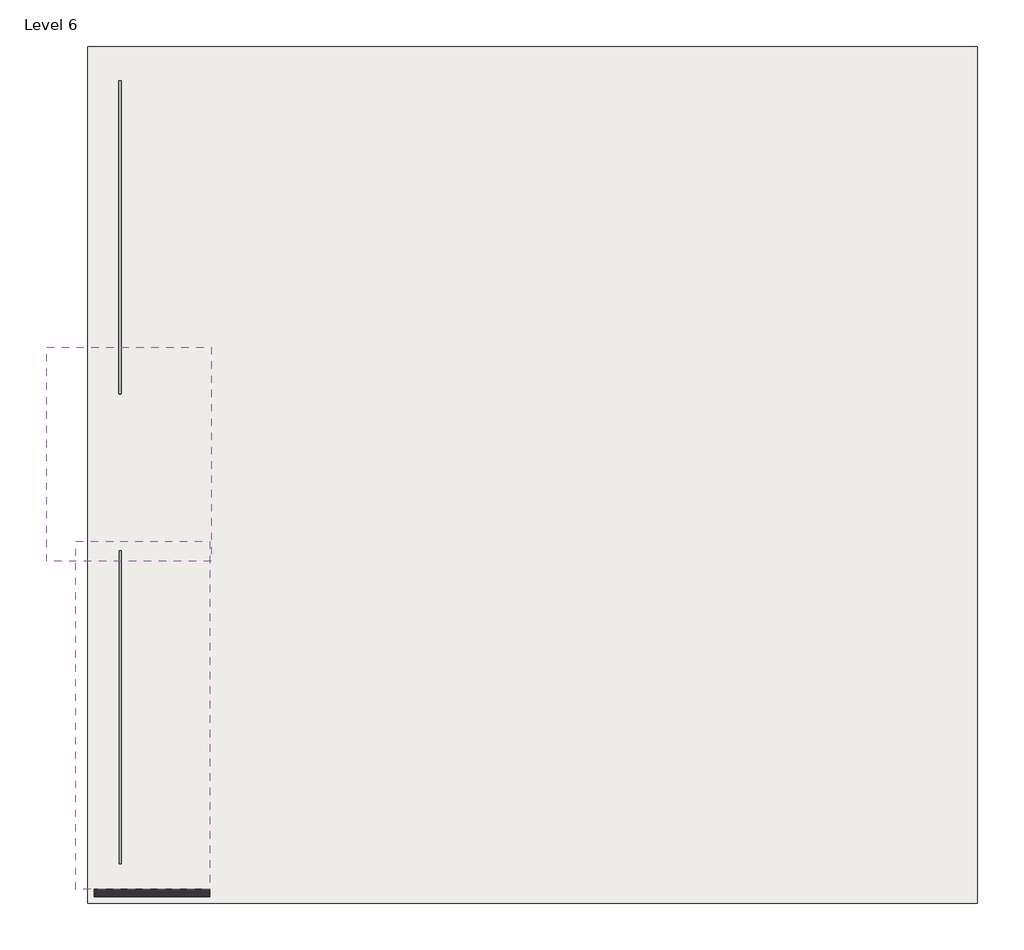
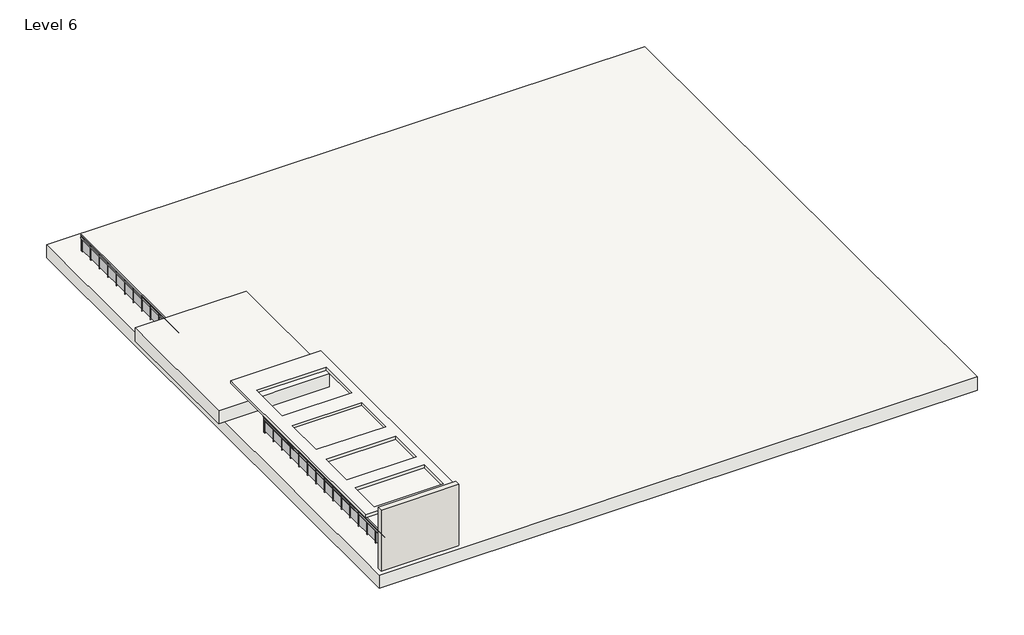
# One storey: 3 slabs, 2 railings, 1 wall.
"""IFC4 building model written with IfcOpenShell, lengths in millimetres."""

from ifc_helpers import new_model, si_unit, point, frame, origin, place, context, project, spatial, polyline, ellipse_curve, trimmed, outline, extrude, element, save
from ifc_brep_helpers import plane_surface, extruded_surface, advanced_brep

model = new_model("IFC4")

# Units and contexts
model_context = context("Model", 3, world=origin())
ifc_project = project(units=[si_unit("LENGTHUNIT", "METRE", prefix="MILLI")], contexts=[model_context])

# Site, building, storey
site = spatial("IfcSite", under=ifc_project)
building = spatial("IfcBuilding", under=site)
storey = spatial("IfcBuildingStorey", under=building, Name="Level 6", Elevation=15240.0)

# Railings
placement = place(None, origin())
element("IfcRailing", 1, ObjectType="Glass Panel - Bottom Fill", at=placement, inside=storey, context=model_context, shape_type="SolidModel", body=[
    advanced_brep(
    [(-15690.0723021, 14300.8556013, 16154.4), (-15766.2723021, 14300.8556013, 16154.4), (-15690.0723021, 2718.4556013, 16154.4), (-15766.2723021, 2718.4556013, 16154.4)],
    [
        (0, 1, ellipse_curve(frame((-15728.1723021, 14300.8556013, 16154.4), z_axis=(0.0, 1.0, 0.0), x_axis=(-1.0, 0.0, 0.0)), 38.1, 28.575)),
        (1, 0, ellipse_curve(frame((-15728.1723021, 14300.8556013, 16154.4), z_axis=(0.0, 1.0, 0.0), x_axis=(-1.0, 0.0, 0.0)), 38.1, 28.575)),
        (2, 3, ellipse_curve(frame((-15728.1723021, 2718.4556013, 16154.4), z_axis=(0.0, -1.0, 0.0), x_axis=(-1.0, 0.0, 0.0)), 38.1, 28.575)),
        (3, 2, ellipse_curve(frame((-15728.1723021, 2718.4556013, 16154.4), z_axis=(0.0, -1.0, 0.0), x_axis=(-1.0, 0.0, 0.0)), 38.1, 28.575)),
        (0, 2),
        (3, 1),
    ],
    [
        plane_surface(frame((-15728.1723021, 14300.8556013, 16154.4), z_axis=(0.0, 1.0, 0.0), x_axis=(0.0, 0.0, -1.0))),
        plane_surface(frame((-15728.1723021, 2718.4556013, 16154.4), z_axis=(0.0, -1.0, 0.0), x_axis=(0.0, 0.0, -1.0))),
        extruded_surface(trimmed(ellipse_curve(frame((-15728.1723021, 2718.4556013, 16154.4), z_axis=(0.0, 1.0, 0.0), x_axis=(-1.0, 0.0, 0.0)), 38.1, 28.575), [point((-15690.0723021, 2718.4556013, 16154.4))], [point((-15766.2723021, 2718.4556013, 16154.4))], True, "CARTESIAN"), (0.0, 11582.4, 0.0), 11582.4),
        extruded_surface(trimmed(ellipse_curve(frame((-15728.1723021, 2718.4556013, 16154.4), z_axis=(0.0, 1.0, 0.0), x_axis=(-1.0, 0.0, 0.0)), 38.1, 28.575), [point((-15766.2723021, 2718.4556013, 16154.4))], [point((-15690.0723021, 2718.4556013, 16154.4))], True, "CARTESIAN"), (0.0, 11582.4, 0.0), 11582.4),
    ],
    [
        (0, [[1, 2]]),
        (1, [[3, 4]]),
        (2, [[-1, 5, -4, 6]]),
        (3, [[-2, -6, -3, -5]]),
    ],
),
    extrude(outline(polyline([(-15753.5723021, 14300.8556013), (-15702.7723021, 14300.8556013), (-15702.7723021, 2718.4556013), (-15753.5723021, 2718.4556013), (-15753.5723021, 14300.8556013)])), frame((0.0, 0.0, 15976.6), z_axis=(0.0, 0.0, 1.0), x_axis=(1.0, 0.0, 0.0)), (0.0, 0.0, 1.0), 76.2),
    extrude(outline(polyline([(-15740.8723021, 14300.8556013), (-15715.4723021, 14300.8556013), (-15715.4723021, 2718.4556013), (-15740.8723021, 2718.4556013), (-15740.8723021, 14300.8556013)])), frame((0.0, 0.0, 15938.5), z_axis=(0.0, 0.0, 1.0), x_axis=(1.0, 0.0, 0.0)), (0.0, 0.0, 1.0), 25.4),
    extrude(outline(polyline([(-15753.5723021, 2826.4056013), (-15702.7723021, 2826.4056013), (-15702.7723021, 2813.7056013), (-15753.5723021, 2813.7056013), (-15753.5723021, 2826.4056013)])), frame((0.0, 0.0, 15240.0), z_axis=(0.0, 0.0, 1.0), x_axis=(1.0, 0.0, 0.0)), (0.0, 0.0, 1.0), 885.6788223),
    extrude(outline(polyline([(-15721.6371451, 3632.8556013), (-15721.6371451, 2820.0556013), (-15727.9871451, 2820.0556013), (-15727.9871451, 3632.8556013), (-15721.6371451, 3632.8556013)])), frame((0.0, 0.0, 15341.6), z_axis=(0.0, 0.0, 1.0), x_axis=(1.0, 0.0, 0.0)), (0.0, 0.0, 1.0), 596.9),
    extrude(outline(polyline([(-15753.5723021, 3639.2056013), (-15702.7723021, 3639.2056013), (-15702.7723021, 3626.5056013), (-15753.5723021, 3626.5056013), (-15753.5723021, 3639.2056013)])), frame((0.0, 0.0, 15240.0), z_axis=(0.0, 0.0, 1.0), x_axis=(1.0, 0.0, 0.0)), (0.0, 0.0, 1.0), 885.6788223),
    extrude(outline(polyline([(-15721.6371451, 4445.6556013), (-15721.6371451, 3632.8556013), (-15727.9871451, 3632.8556013), (-15727.9871451, 4445.6556013), (-15721.6371451, 4445.6556013)])), frame((0.0, 0.0, 15341.6), z_axis=(0.0, 0.0, 1.0), x_axis=(1.0, 0.0, 0.0)), (0.0, 0.0, 1.0), 596.9),
    extrude(outline(polyline([(-15753.5723021, 4452.0056013), (-15702.7723021, 4452.0056013), (-15702.7723021, 4439.3056013), (-15753.5723021, 4439.3056013), (-15753.5723021, 4452.0056013)])), frame((0.0, 0.0, 15240.0), z_axis=(0.0, 0.0, 1.0), x_axis=(1.0, 0.0, 0.0)), (0.0, 0.0, 1.0), 885.6788223),
    extrude(outline(polyline([(-15721.6371451, 5258.4556013), (-15721.6371451, 4445.6556013), (-15727.9871451, 4445.6556013), (-15727.9871451, 5258.4556013), (-15721.6371451, 5258.4556013)])), frame((0.0, 0.0, 15341.6), z_axis=(0.0, 0.0, 1.0), x_axis=(1.0, 0.0, 0.0)), (0.0, 0.0, 1.0), 596.9),
    extrude(outline(polyline([(-15753.5723021, 5264.8056013), (-15702.7723021, 5264.8056013), (-15702.7723021, 5252.1056013), (-15753.5723021, 5252.1056013), (-15753.5723021, 5264.8056013)])), frame((0.0, 0.0, 15240.0), z_axis=(0.0, 0.0, 1.0), x_axis=(1.0, 0.0, 0.0)), (0.0, 0.0, 1.0), 885.6788223),
    extrude(outline(polyline([(-15721.6371451, 6071.2556013), (-15721.6371451, 5258.4556013), (-15727.9871451, 5258.4556013), (-15727.9871451, 6071.2556013), (-15721.6371451, 6071.2556013)])), frame((0.0, 0.0, 15341.6), z_axis=(0.0, 0.0, 1.0), x_axis=(1.0, 0.0, 0.0)), (0.0, 0.0, 1.0), 596.9),
    extrude(outline(polyline([(-15753.5723021, 6077.6056013), (-15702.7723021, 6077.6056013), (-15702.7723021, 6064.9056013), (-15753.5723021, 6064.9056013), (-15753.5723021, 6077.6056013)])), frame((0.0, 0.0, 15240.0), z_axis=(0.0, 0.0, 1.0), x_axis=(1.0, 0.0, 0.0)), (0.0, 0.0, 1.0), 885.6788223),
    extrude(outline(polyline([(-15721.6371451, 6884.0556013), (-15721.6371451, 6071.2556013), (-15727.9871451, 6071.2556013), (-15727.9871451, 6884.0556013), (-15721.6371451, 6884.0556013)])), frame((0.0, 0.0, 15341.6), z_axis=(0.0, 0.0, 1.0), x_axis=(1.0, 0.0, 0.0)), (0.0, 0.0, 1.0), 596.9),
    extrude(outline(polyline([(-15753.5723021, 6890.4056013), (-15702.7723021, 6890.4056013), (-15702.7723021, 6877.7056013), (-15753.5723021, 6877.7056013), (-15753.5723021, 6890.4056013)])), frame((0.0, 0.0, 15240.0), z_axis=(0.0, 0.0, 1.0), x_axis=(1.0, 0.0, 0.0)), (0.0, 0.0, 1.0), 885.6788223),
    extrude(outline(polyline([(-15721.6371451, 7696.8556013), (-15721.6371451, 6884.0556013), (-15727.9871451, 6884.0556013), (-15727.9871451, 7696.8556013), (-15721.6371451, 7696.8556013)])), frame((0.0, 0.0, 15341.6), z_axis=(0.0, 0.0, 1.0), x_axis=(1.0, 0.0, 0.0)), (0.0, 0.0, 1.0), 596.9),
    extrude(outline(polyline([(-15753.5723021, 7703.2056013), (-15702.7723021, 7703.2056013), (-15702.7723021, 7690.5056013), (-15753.5723021, 7690.5056013), (-15753.5723021, 7703.2056013)])), frame((0.0, 0.0, 15240.0), z_axis=(0.0, 0.0, 1.0), x_axis=(1.0, 0.0, 0.0)), (0.0, 0.0, 1.0), 885.6788223),
    extrude(outline(polyline([(-15721.6371451, 8509.6556013), (-15721.6371451, 7696.8556013), (-15727.9871451, 7696.8556013), (-15727.9871451, 8509.6556013), (-15721.6371451, 8509.6556013)])), frame((0.0, 0.0, 15341.6), z_axis=(0.0, 0.0, 1.0), x_axis=(1.0, 0.0, 0.0)), (0.0, 0.0, 1.0), 596.9),
    extrude(outline(polyline([(-15753.5723021, 8516.0056013), (-15702.7723021, 8516.0056013), (-15702.7723021, 8503.3056013), (-15753.5723021, 8503.3056013), (-15753.5723021, 8516.0056013)])), frame((0.0, 0.0, 15240.0), z_axis=(0.0, 0.0, 1.0), x_axis=(1.0, 0.0, 0.0)), (0.0, 0.0, 1.0), 885.6788223),
    extrude(outline(polyline([(-15721.6371451, 9322.4556013), (-15721.6371451, 8509.6556013), (-15727.9871451, 8509.6556013), (-15727.9871451, 9322.4556013), (-15721.6371451, 9322.4556013)])), frame((0.0, 0.0, 15341.6), z_axis=(0.0, 0.0, 1.0), x_axis=(1.0, 0.0, 0.0)), (0.0, 0.0, 1.0), 596.9),
    extrude(outline(polyline([(-15753.5723021, 9328.8056013), (-15702.7723021, 9328.8056013), (-15702.7723021, 9316.1056013), (-15753.5723021, 9316.1056013), (-15753.5723021, 9328.8056013)])), frame((0.0, 0.0, 15240.0), z_axis=(0.0, 0.0, 1.0), x_axis=(1.0, 0.0, 0.0)), (0.0, 0.0, 1.0), 885.6788223),
    extrude(outline(polyline([(-15721.6371451, 10135.2556013), (-15721.6371451, 9322.4556013), (-15727.9871451, 9322.4556013), (-15727.9871451, 10135.2556013), (-15721.6371451, 10135.2556013)])), frame((0.0, 0.0, 15341.6), z_axis=(0.0, 0.0, 1.0), x_axis=(1.0, 0.0, 0.0)), (0.0, 0.0, 1.0), 596.9),
    extrude(outline(polyline([(-15753.5723021, 10141.6056013), (-15702.7723021, 10141.6056013), (-15702.7723021, 10128.9056013), (-15753.5723021, 10128.9056013), (-15753.5723021, 10141.6056013)])), frame((0.0, 0.0, 15240.0), z_axis=(0.0, 0.0, 1.0), x_axis=(1.0, 0.0, 0.0)), (0.0, 0.0, 1.0), 885.6788223),
    extrude(outline(polyline([(-15721.6371451, 10948.0556013), (-15721.6371451, 10135.2556013), (-15727.9871451, 10135.2556013), (-15727.9871451, 10948.0556013), (-15721.6371451, 10948.0556013)])), frame((0.0, 0.0, 15341.6), z_axis=(0.0, 0.0, 1.0), x_axis=(1.0, 0.0, 0.0)), (0.0, 0.0, 1.0), 596.9),
    extrude(outline(polyline([(-15753.5723021, 10954.4056013), (-15702.7723021, 10954.4056013), (-15702.7723021, 10941.7056013), (-15753.5723021, 10941.7056013), (-15753.5723021, 10954.4056013)])), frame((0.0, 0.0, 15240.0), z_axis=(0.0, 0.0, 1.0), x_axis=(1.0, 0.0, 0.0)), (0.0, 0.0, 1.0), 885.6788223),
    extrude(outline(polyline([(-15721.6371451, 11760.8556013), (-15721.6371451, 10948.0556013), (-15727.9871451, 10948.0556013), (-15727.9871451, 11760.8556013), (-15721.6371451, 11760.8556013)])), frame((0.0, 0.0, 15341.6), z_axis=(0.0, 0.0, 1.0), x_axis=(1.0, 0.0, 0.0)), (0.0, 0.0, 1.0), 596.9),
    extrude(outline(polyline([(-15753.5723021, 11767.2056013), (-15702.7723021, 11767.2056013), (-15702.7723021, 11754.5056013), (-15753.5723021, 11754.5056013), (-15753.5723021, 11767.2056013)])), frame((0.0, 0.0, 15240.0), z_axis=(0.0, 0.0, 1.0), x_axis=(1.0, 0.0, 0.0)), (0.0, 0.0, 1.0), 885.6788223),
    extrude(outline(polyline([(-15721.6371451, 12573.6556013), (-15721.6371451, 11760.8556013), (-15727.9871451, 11760.8556013), (-15727.9871451, 12573.6556013), (-15721.6371451, 12573.6556013)])), frame((0.0, 0.0, 15341.6), z_axis=(0.0, 0.0, 1.0), x_axis=(1.0, 0.0, 0.0)), (0.0, 0.0, 1.0), 596.9),
    extrude(outline(polyline([(-15753.5723021, 12580.0056013), (-15702.7723021, 12580.0056013), (-15702.7723021, 12567.3056013), (-15753.5723021, 12567.3056013), (-15753.5723021, 12580.0056013)])), frame((0.0, 0.0, 15240.0), z_axis=(0.0, 0.0, 1.0), x_axis=(1.0, 0.0, 0.0)), (0.0, 0.0, 1.0), 885.6788223),
    extrude(outline(polyline([(-15721.6371451, 13386.4556013), (-15721.6371451, 12573.6556013), (-15727.9871451, 12573.6556013), (-15727.9871451, 13386.4556013), (-15721.6371451, 13386.4556013)])), frame((0.0, 0.0, 15341.6), z_axis=(0.0, 0.0, 1.0), x_axis=(1.0, 0.0, 0.0)), (0.0, 0.0, 1.0), 596.9),
    extrude(outline(polyline([(-15753.5723021, 13392.8056013), (-15702.7723021, 13392.8056013), (-15702.7723021, 13380.1056013), (-15753.5723021, 13380.1056013), (-15753.5723021, 13392.8056013)])), frame((0.0, 0.0, 15240.0), z_axis=(0.0, 0.0, 1.0), x_axis=(1.0, 0.0, 0.0)), (0.0, 0.0, 1.0), 885.6788223),
    extrude(outline(polyline([(-15721.6371451, 14199.2556013), (-15721.6371451, 13386.4556013), (-15727.9871451, 13386.4556013), (-15727.9871451, 14199.2556013), (-15721.6371451, 14199.2556013)])), frame((0.0, 0.0, 15341.6), z_axis=(0.0, 0.0, 1.0), x_axis=(1.0, 0.0, 0.0)), (0.0, 0.0, 1.0), 596.9),
    extrude(outline(polyline([(-15753.5723021, 14205.6056013), (-15702.7723021, 14205.6056013), (-15702.7723021, 14192.9056013), (-15753.5723021, 14192.9056013), (-15753.5723021, 14205.6056013)])), frame((0.0, 0.0, 15240.0), z_axis=(0.0, 0.0, 1.0), x_axis=(1.0, 0.0, 0.0)), (0.0, 0.0, 1.0), 885.6788223),
    extrude(outline(polyline([(-15737.6973021, 2731.1556013), (-15718.6473021, 2731.1556013), (-15718.6473021, 2712.1056013), (-15737.6973021, 2712.1056013), (-15737.6973021, 2731.1556013)])), frame((0.0, 0.0, 15240.0), z_axis=(0.0, 0.0, 1.0), x_axis=(1.0, 0.0, 0.0)), (0.0, 0.0, 1.0), 885.6788223),
    extrude(outline(polyline([(-15737.6973021, 14307.2056013), (-15718.6473021, 14307.2056013), (-15718.6473021, 14288.1556013), (-15737.6973021, 14288.1556013), (-15737.6973021, 14307.2056013)])), frame((0.0, 0.0, 15240.0), z_axis=(0.0, 0.0, 1.0), x_axis=(1.0, 0.0, 0.0)), (0.0, 0.0, 1.0), 885.6788223),
])
element("IfcRailing", 2, ObjectType="Glass Panel - Bottom Fill", at=placement, inside=storey, context=model_context, shape_type="SolidModel", body=[
    advanced_brep(
    [(-15683.0239142, -3085.7495575, 16154.4), (-15759.2239142, -3085.7495575, 16154.4), (-15683.0239142, -14668.1495575, 16154.4), (-15759.2239142, -14668.1495575, 16154.4)],
    [
        (0, 1, ellipse_curve(frame((-15721.1239142, -3085.7495575, 16154.4), z_axis=(0.0, 1.0, 0.0), x_axis=(-1.0, 0.0, 0.0)), 38.1, 28.575)),
        (1, 0, ellipse_curve(frame((-15721.1239142, -3085.7495575, 16154.4), z_axis=(0.0, 1.0, 0.0), x_axis=(-1.0, 0.0, 0.0)), 38.1, 28.575)),
        (2, 3, ellipse_curve(frame((-15721.1239142, -14668.1495575, 16154.4), z_axis=(0.0, -1.0, 0.0), x_axis=(-1.0, 0.0, 0.0)), 38.1, 28.575)),
        (3, 2, ellipse_curve(frame((-15721.1239142, -14668.1495575, 16154.4), z_axis=(0.0, -1.0, 0.0), x_axis=(-1.0, 0.0, 0.0)), 38.1, 28.575)),
        (0, 2),
        (3, 1),
    ],
    [
        plane_surface(frame((-15721.1239142, -3085.7495575, 16154.4), z_axis=(0.0, 1.0, 0.0), x_axis=(0.0, 0.0, -1.0))),
        plane_surface(frame((-15721.1239142, -14668.1495575, 16154.4), z_axis=(0.0, -1.0, 0.0), x_axis=(0.0, 0.0, -1.0))),
        extruded_surface(trimmed(ellipse_curve(frame((-15721.1239142, -14668.1495575, 16154.4), z_axis=(0.0, 1.0, 0.0), x_axis=(-1.0, 0.0, 0.0)), 38.1, 28.575), [point((-15683.0239142, -14668.1495575, 16154.4))], [point((-15759.2239142, -14668.1495575, 16154.4))], True, "CARTESIAN"), (0.0, 11582.400000000001, 0.0), 11582.400000000001),
        extruded_surface(trimmed(ellipse_curve(frame((-15721.1239142, -14668.1495575, 16154.4), z_axis=(0.0, 1.0, 0.0), x_axis=(-1.0, 0.0, 0.0)), 38.1, 28.575), [point((-15759.2239142, -14668.1495575, 16154.4))], [point((-15683.0239142, -14668.1495575, 16154.4))], True, "CARTESIAN"), (0.0, 11582.400000000001, 0.0), 11582.400000000001),
    ],
    [
        (0, [[1, 2]]),
        (1, [[3, 4]]),
        (2, [[-1, 5, -4, 6]]),
        (3, [[-2, -6, -3, -5]]),
    ],
),
    extrude(outline(polyline([(-15746.5239142, -3085.7495575), (-15695.7239142, -3085.7495575), (-15695.7239142, -14668.1495575), (-15746.5239142, -14668.1495575), (-15746.5239142, -3085.7495575)])), frame((0.0, 0.0, 15976.6), z_axis=(0.0, 0.0, 1.0), x_axis=(1.0, 0.0, 0.0)), (0.0, 0.0, 1.0), 76.2),
    extrude(outline(polyline([(-15733.8239142, -3085.7495575), (-15708.4239142, -3085.7495575), (-15708.4239142, -14668.1495575), (-15733.8239142, -14668.1495575), (-15733.8239142, -3085.7495575)])), frame((0.0, 0.0, 15938.5), z_axis=(0.0, 0.0, 1.0), x_axis=(1.0, 0.0, 0.0)), (0.0, 0.0, 1.0), 25.4),
    extrude(outline(polyline([(-15746.5239142, -14560.1995575), (-15695.7239142, -14560.1995575), (-15695.7239142, -14572.8995575), (-15746.5239142, -14572.8995575), (-15746.5239142, -14560.1995575)])), frame((0.0, 0.0, 15240.0), z_axis=(0.0, 0.0, 1.0), x_axis=(1.0, 0.0, 0.0)), (0.0, 0.0, 1.0), 885.6788223),
    extrude(outline(polyline([(-15714.5887572, -13753.7495575), (-15714.5887572, -14566.5495575), (-15720.9387572, -14566.5495575), (-15720.9387572, -13753.7495575), (-15714.5887572, -13753.7495575)])), frame((0.0, 0.0, 15341.6), z_axis=(0.0, 0.0, 1.0), x_axis=(1.0, 0.0, 0.0)), (0.0, 0.0, 1.0), 596.9),
    extrude(outline(polyline([(-15746.5239142, -13747.3995575), (-15695.7239142, -13747.3995575), (-15695.7239142, -13760.0995575), (-15746.5239142, -13760.0995575), (-15746.5239142, -13747.3995575)])), frame((0.0, 0.0, 15240.0), z_axis=(0.0, 0.0, 1.0), x_axis=(1.0, 0.0, 0.0)), (0.0, 0.0, 1.0), 885.6788223),
    extrude(outline(polyline([(-15714.5887572, -12940.9495575), (-15714.5887572, -13753.7495575), (-15720.9387572, -13753.7495575), (-15720.9387572, -12940.9495575), (-15714.5887572, -12940.9495575)])), frame((0.0, 0.0, 15341.6), z_axis=(0.0, 0.0, 1.0), x_axis=(1.0, 0.0, 0.0)), (0.0, 0.0, 1.0), 596.9),
    extrude(outline(polyline([(-15746.5239142, -12934.5995575), (-15695.7239142, -12934.5995575), (-15695.7239142, -12947.2995575), (-15746.5239142, -12947.2995575), (-15746.5239142, -12934.5995575)])), frame((0.0, 0.0, 15240.0), z_axis=(0.0, 0.0, 1.0), x_axis=(1.0, 0.0, 0.0)), (0.0, 0.0, 1.0), 885.6788223),
    extrude(outline(polyline([(-15714.5887572, -12128.1495575), (-15714.5887572, -12940.9495575), (-15720.9387572, -12940.9495575), (-15720.9387572, -12128.1495575), (-15714.5887572, -12128.1495575)])), frame((0.0, 0.0, 15341.6), z_axis=(0.0, 0.0, 1.0), x_axis=(1.0, 0.0, 0.0)), (0.0, 0.0, 1.0), 596.9),
    extrude(outline(polyline([(-15746.5239142, -12121.7995575), (-15695.7239142, -12121.7995575), (-15695.7239142, -12134.4995575), (-15746.5239142, -12134.4995575), (-15746.5239142, -12121.7995575)])), frame((0.0, 0.0, 15240.0), z_axis=(0.0, 0.0, 1.0), x_axis=(1.0, 0.0, 0.0)), (0.0, 0.0, 1.0), 885.6788223),
    extrude(outline(polyline([(-15714.5887572, -11315.3495575), (-15714.5887572, -12128.1495575), (-15720.9387572, -12128.1495575), (-15720.9387572, -11315.3495575), (-15714.5887572, -11315.3495575)])), frame((0.0, 0.0, 15341.6), z_axis=(0.0, 0.0, 1.0), x_axis=(1.0, 0.0, 0.0)), (0.0, 0.0, 1.0), 596.9),
    extrude(outline(polyline([(-15746.5239142, -11308.9995575), (-15695.7239142, -11308.9995575), (-15695.7239142, -11321.6995575), (-15746.5239142, -11321.6995575), (-15746.5239142, -11308.9995575)])), frame((0.0, 0.0, 15240.0), z_axis=(0.0, 0.0, 1.0), x_axis=(1.0, 0.0, 0.0)), (0.0, 0.0, 1.0), 885.6788223),
    extrude(outline(polyline([(-15714.5887572, -10502.5495575), (-15714.5887572, -11315.3495575), (-15720.9387572, -11315.3495575), (-15720.9387572, -10502.5495575), (-15714.5887572, -10502.5495575)])), frame((0.0, 0.0, 15341.6), z_axis=(0.0, 0.0, 1.0), x_axis=(1.0, 0.0, 0.0)), (0.0, 0.0, 1.0), 596.9),
    extrude(outline(polyline([(-15746.5239142, -10496.1995575), (-15695.7239142, -10496.1995575), (-15695.7239142, -10508.8995575), (-15746.5239142, -10508.8995575), (-15746.5239142, -10496.1995575)])), frame((0.0, 0.0, 15240.0), z_axis=(0.0, 0.0, 1.0), x_axis=(1.0, 0.0, 0.0)), (0.0, 0.0, 1.0), 885.6788223),
    extrude(outline(polyline([(-15714.5887572, -9689.7495575), (-15714.5887572, -10502.5495575), (-15720.9387572, -10502.5495575), (-15720.9387572, -9689.7495575), (-15714.5887572, -9689.7495575)])), frame((0.0, 0.0, 15341.6), z_axis=(0.0, 0.0, 1.0), x_axis=(1.0, 0.0, 0.0)), (0.0, 0.0, 1.0), 596.9),
    extrude(outline(polyline([(-15746.5239142, -9683.3995575), (-15695.7239142, -9683.3995575), (-15695.7239142, -9696.0995575), (-15746.5239142, -9696.0995575), (-15746.5239142, -9683.3995575)])), frame((0.0, 0.0, 15240.0), z_axis=(0.0, 0.0, 1.0), x_axis=(1.0, 0.0, 0.0)), (0.0, 0.0, 1.0), 885.6788223),
    extrude(outline(polyline([(-15714.5887572, -8876.9495575), (-15714.5887572, -9689.7495575), (-15720.9387572, -9689.7495575), (-15720.9387572, -8876.9495575), (-15714.5887572, -8876.9495575)])), frame((0.0, 0.0, 15341.6), z_axis=(0.0, 0.0, 1.0), x_axis=(1.0, 0.0, 0.0)), (0.0, 0.0, 1.0), 596.9),
    extrude(outline(polyline([(-15746.5239142, -8870.5995575), (-15695.7239142, -8870.5995575), (-15695.7239142, -8883.2995575), (-15746.5239142, -8883.2995575), (-15746.5239142, -8870.5995575)])), frame((0.0, 0.0, 15240.0), z_axis=(0.0, 0.0, 1.0), x_axis=(1.0, 0.0, 0.0)), (0.0, 0.0, 1.0), 885.6788223),
    extrude(outline(polyline([(-15714.5887572, -8064.1495575), (-15714.5887572, -8876.9495575), (-15720.9387572, -8876.9495575), (-15720.9387572, -8064.1495575), (-15714.5887572, -8064.1495575)])), frame((0.0, 0.0, 15341.6), z_axis=(0.0, 0.0, 1.0), x_axis=(1.0, 0.0, 0.0)), (0.0, 0.0, 1.0), 596.9),
    extrude(outline(polyline([(-15746.5239142, -8057.7995575), (-15695.7239142, -8057.7995575), (-15695.7239142, -8070.4995575), (-15746.5239142, -8070.4995575), (-15746.5239142, -8057.7995575)])), frame((0.0, 0.0, 15240.0), z_axis=(0.0, 0.0, 1.0), x_axis=(1.0, 0.0, 0.0)), (0.0, 0.0, 1.0), 885.6788223),
    extrude(outline(polyline([(-15714.5887572, -7251.3495575), (-15714.5887572, -8064.1495575), (-15720.9387572, -8064.1495575), (-15720.9387572, -7251.3495575), (-15714.5887572, -7251.3495575)])), frame((0.0, 0.0, 15341.6), z_axis=(0.0, 0.0, 1.0), x_axis=(1.0, 0.0, 0.0)), (0.0, 0.0, 1.0), 596.9),
    extrude(outline(polyline([(-15746.5239142, -7244.9995575), (-15695.7239142, -7244.9995575), (-15695.7239142, -7257.6995575), (-15746.5239142, -7257.6995575), (-15746.5239142, -7244.9995575)])), frame((0.0, 0.0, 15240.0), z_axis=(0.0, 0.0, 1.0), x_axis=(1.0, 0.0, 0.0)), (0.0, 0.0, 1.0), 885.6788223),
    extrude(outline(polyline([(-15714.5887572, -6438.5495575), (-15714.5887572, -7251.3495575), (-15720.9387572, -7251.3495575), (-15720.9387572, -6438.5495575), (-15714.5887572, -6438.5495575)])), frame((0.0, 0.0, 15341.6), z_axis=(0.0, 0.0, 1.0), x_axis=(1.0, 0.0, 0.0)), (0.0, 0.0, 1.0), 596.9),
    extrude(outline(polyline([(-15746.5239142, -6432.1995575), (-15695.7239142, -6432.1995575), (-15695.7239142, -6444.8995575), (-15746.5239142, -6444.8995575), (-15746.5239142, -6432.1995575)])), frame((0.0, 0.0, 15240.0), z_axis=(0.0, 0.0, 1.0), x_axis=(1.0, 0.0, 0.0)), (0.0, 0.0, 1.0), 885.6788223),
    extrude(outline(polyline([(-15714.5887572, -5625.7495575), (-15714.5887572, -6438.5495575), (-15720.9387572, -6438.5495575), (-15720.9387572, -5625.7495575), (-15714.5887572, -5625.7495575)])), frame((0.0, 0.0, 15341.6), z_axis=(0.0, 0.0, 1.0), x_axis=(1.0, 0.0, 0.0)), (0.0, 0.0, 1.0), 596.9),
    extrude(outline(polyline([(-15746.5239142, -5619.3995575), (-15695.7239142, -5619.3995575), (-15695.7239142, -5632.0995575), (-15746.5239142, -5632.0995575), (-15746.5239142, -5619.3995575)])), frame((0.0, 0.0, 15240.0), z_axis=(0.0, 0.0, 1.0), x_axis=(1.0, 0.0, 0.0)), (0.0, 0.0, 1.0), 885.6788223),
    extrude(outline(polyline([(-15714.5887572, -4812.9495575), (-15714.5887572, -5625.7495575), (-15720.9387572, -5625.7495575), (-15720.9387572, -4812.9495575), (-15714.5887572, -4812.9495575)])), frame((0.0, 0.0, 15341.6), z_axis=(0.0, 0.0, 1.0), x_axis=(1.0, 0.0, 0.0)), (0.0, 0.0, 1.0), 596.9),
    extrude(outline(polyline([(-15746.5239142, -4806.5995575), (-15695.7239142, -4806.5995575), (-15695.7239142, -4819.2995575), (-15746.5239142, -4819.2995575), (-15746.5239142, -4806.5995575)])), frame((0.0, 0.0, 15240.0), z_axis=(0.0, 0.0, 1.0), x_axis=(1.0, 0.0, 0.0)), (0.0, 0.0, 1.0), 885.6788223),
    extrude(outline(polyline([(-15714.5887572, -4000.1495575), (-15714.5887572, -4812.9495575), (-15720.9387572, -4812.9495575), (-15720.9387572, -4000.1495575), (-15714.5887572, -4000.1495575)])), frame((0.0, 0.0, 15341.6), z_axis=(0.0, 0.0, 1.0), x_axis=(1.0, 0.0, 0.0)), (0.0, 0.0, 1.0), 596.9),
    extrude(outline(polyline([(-15746.5239142, -3993.7995575), (-15695.7239142, -3993.7995575), (-15695.7239142, -4006.4995575), (-15746.5239142, -4006.4995575), (-15746.5239142, -3993.7995575)])), frame((0.0, 0.0, 15240.0), z_axis=(0.0, 0.0, 1.0), x_axis=(1.0, 0.0, 0.0)), (0.0, 0.0, 1.0), 885.6788223),
    extrude(outline(polyline([(-15714.5887572, -3187.3495575), (-15714.5887572, -4000.1495575), (-15720.9387572, -4000.1495575), (-15720.9387572, -3187.3495575), (-15714.5887572, -3187.3495575)])), frame((0.0, 0.0, 15341.6), z_axis=(0.0, 0.0, 1.0), x_axis=(1.0, 0.0, 0.0)), (0.0, 0.0, 1.0), 596.9),
    extrude(outline(polyline([(-15746.5239142, -3180.9995575), (-15695.7239142, -3180.9995575), (-15695.7239142, -3193.6995575), (-15746.5239142, -3193.6995575), (-15746.5239142, -3180.9995575)])), frame((0.0, 0.0, 15240.0), z_axis=(0.0, 0.0, 1.0), x_axis=(1.0, 0.0, 0.0)), (0.0, 0.0, 1.0), 885.6788223),
    extrude(outline(polyline([(-15730.6489142, -14655.4495575), (-15711.5989142, -14655.4495575), (-15711.5989142, -14674.4995575), (-15730.6489142, -14674.4995575), (-15730.6489142, -14655.4495575)])), frame((0.0, 0.0, 15240.0), z_axis=(0.0, 0.0, 1.0), x_axis=(1.0, 0.0, 0.0)), (0.0, 0.0, 1.0), 885.6788223),
    extrude(outline(polyline([(-15730.6489142, -3079.3995575), (-15711.5989142, -3079.3995575), (-15711.5989142, -3098.4495575), (-15730.6489142, -3098.4495575), (-15730.6489142, -3079.3995575)])), frame((0.0, 0.0, 15240.0), z_axis=(0.0, 0.0, 1.0), x_axis=(1.0, 0.0, 0.0)), (0.0, 0.0, 1.0), 885.6788223),
])

# Slabs
element("IfcSlab", 3, ObjectType="Generic - 12\"", at=placement, inside=storey, context=model_context, shape_type="SweptSolid", body=[
    extrude(outline(polyline([(-12350.7244174, 4446.2532825), (-12350.7244174, -3478.5467175), (-18446.7244174, -3478.5467175), (-18446.7244174, 4446.2532825), (-12350.7244174, 4446.2532825)])), frame((0.0, 0.0, 16916.4), z_axis=(0.0, 0.0, 1.0), x_axis=(1.0, 0.0, 0.0)), (0.0, 0.0, 1.0), 762.0),
])
element("IfcSlab", 4, ObjectType="Generic - 12\"", at=placement, inside=storey, context=model_context, shape_type="SweptSolid", body=[
    extrude(outline(polyline([(16005.4811212, 15572.3906851), (16005.4811212, -16126.8093149), (-16912.9188788, -16126.8093149), (-16912.9188788, 15572.3906851), (16005.4811212, 15572.3906851)])), frame((0.0, 0.0, 14478.0), z_axis=(0.0, 0.0, 1.0), x_axis=(1.0, 0.0, 0.0)), (0.0, 0.0, 1.0), 762.0),
])
element("IfcSlab", 5, ObjectType="f1", at=placement, inside=storey, context=model_context, shape_type="SweptSolid", body=[
    extrude(outline(polyline([(-12413.4723021, -2742.5443987), (-12413.4723021, -15620.3443987), (-17358.737313, -15620.3443987), (-17358.737313, -2742.5443987), (-12413.4723021, -2742.5443987)]), holes=[polyline([(-12870.6723021, -4062.2708755), (-16680.6723021, -4062.2708755), (-16680.6723021, -6500.6708755), (-12870.6723021, -6500.6708755), (-12870.6723021, -4062.2708755)]), polyline([(-12870.6723021, -7459.6975553), (-16680.6723021, -7459.6975553), (-16680.6723021, -9739.2892328), (-12870.6723021, -9739.2892328), (-12870.6723021, -7459.6975553)]), polyline([(-12870.6723021, -10687.6071774), (-16680.6723021, -10687.6071774), (-16680.6723021, -12657.2823534), (-12870.6723021, -12657.2823534), (-12870.6723021, -10687.6071774)]), polyline([(-12870.6723021, -13425.939386), (-16680.6723021, -13425.939386), (-16680.6723021, -15237.6629151), (-12870.6723021, -15237.6629151), (-12870.6723021, -13425.939386)])]), frame((0.0, 0.0, 18440.4), z_axis=(0.0, 0.0, 1.0), x_axis=(1.0, 0.0, 0.0)), (0.0, 0.0, 1.0), 152.4),
])

# Wall
element("IfcWall", 6, ObjectType="ext", at=placement, inside=storey, context=model_context, shape_type="SweptSolid", body=[
    extrude(outline(polyline([(-12413.4723021, -15899.7443987), (-16680.6723021, -15899.7443987), (-16680.6723021, -15620.3443987), (-12413.4723021, -15620.3443987), (-12413.4723021, -15899.7443987)])), frame((0.0, 0.0, 15240.0), z_axis=(0.0, 0.0, 1.0), x_axis=(1.0, 0.0, 0.0)), (0.0, 0.0, 1.0), 3567.8965807),
])

save(model, "model.ifc")

# Revit data of these elements
# Type "Glass Panel - Bottom Fill"
#   Assembly Code = "C2010400"
#   built-in parameter 1008612 = 0.0416667 (stored number, unit not read)
#   built-in parameter 1008611 = 0.0416667 (stored number, unit not read)
#   built-in parameter 1008609 = 0.333333 (stored number, unit not read)
#   built-in parameter 1008604 = 0.166667 (stored number, unit not read)
#   built-in parameter 1008603 = 0.166667 (stored number, unit not read)
#   Railing Height = 3' - 0"
#   built-in parameter 1008631 = 1
#   built-in parameter 1008630 = 2
#   built-in parameter 1008610 = 2
#   built-in parameter 1008618 = Baluster - Square : 3/4"
# Type "Generic - 12\""
#   Assembly Code = "B1010"
#   Function = 0
#   Layers, outside or top first: 2' - 6" no material (function 1)
# Type "f1"
#   Assembly Code = "B1010"
#   Function = 0
#   Layers, outside or top first: 0' - 6" no material (function 1)
# Type "ext"
#   Assembly Code = "B2010"
#   Layers, outside or top first: 0' - 11" "Acoustic Ceiling Tile 24 x 24" (function 1)
# Elements 1, 2 (IfcRailing, "Glass Panel - Bottom Fill")
#   Phase Created = New Construction
#   Materials on its faces: "Glass"
# Element 3 (IfcSlab, "Generic - 12\"")
#   Height Offset From Level = 8' - 0"
#   Phase Created = New Construction
#   Materials on its faces: "Default Floor"
# Element 4 (IfcSlab, "Generic - 12\"")
#   Height Offset From Level = 0' - 0"
#   Phase Created = New Construction
#   Materials on its faces: "Default Floor"
# Element 5 (IfcSlab, "f1")
#   Height Offset From Level = 11' - 0"
#   Phase Created = New Construction
#   Materials on its faces: "Default Floor"
# Element 6 (IfcWall, "ext")
#   Top Offset = 0' - 0"
#   Base Offset = 0' - 0"
#   Unconnected Height = 11' - 8.46837"
#   wall height = 11' - 8.46837"
#   Phase Created = New Construction
#   Base Constraint = Level 6
#   Materials on its faces: "Acoustic Ceiling Tile 24 x 24"
# Materials
#   "Acoustic Ceiling Tile 24 x 24": class "Generic", colour RGB 232 232 232, transparency 0, Description = "Acoustic Ceiling Tile 24 x 24", Cost = 0
#   "Glass": class "Glass", colour RGB 0 128 192, transparency 0.75, Description = "Soda Lime Glass", Cost = 0
#   "Default Floor": colour RGB 128 128 128, transparency 0
